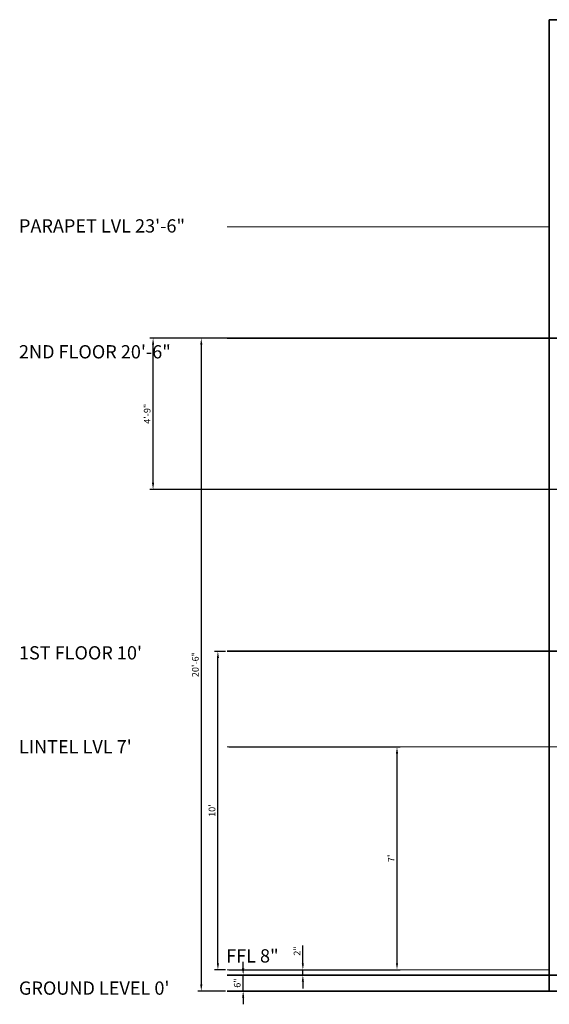
# Model space of a CAD drawing. Units: inches. Extents: x 2443635 to 2446153, y 1826255 to 1827341.
# Tile 12 of 16: x 2444943 to 2445143, y 1826858 to 1827229. Entities that reach past the tile are written whole.
import ezdxf

# ---------------------------------------------------------------- set-up
doc = ezdxf.new("R2010")
doc.units = ezdxf.units.IN
for name, color, linetype, lineweight in [('A-ANNO-LEVL', 4, 'Continuous', 18), ('A-DIMS', 1, 'Continuous', 18), ('A-SECT', 7, 'Continuous', 35)]:
    doc.layers.add(name, color=color, linetype=linetype, lineweight=lineweight)
doc.styles.get("Standard").update_dxf_attribs({"font": 'arial.ttf'})
doc.dimstyles.new('ISO-25', dxfattribs={"dimtxt": 2.5, "dimasz": 2.5, "dimexe": 1.25, "dimexo": 0.625, "dimtad": 1, "dimlunit": 4, "dimtxsty": 'Standard', "dimcen": 2.5, "dimadec": 0, "dimazin": 0, "dimtfac": 1, "dimtmove": 0, "dimatfit": 3, "dimfxl": 1, "dimarcsym": 0})

# ---------------------------------------------------------------- blocks, each defined once
blk = doc.blocks.new('*D31')
at = {"layer": 'A-DIMS', "color": 0, "lineweight": -2, "transparency": 16777216}
for p, q in [((2445027.46, 1826871.2), (2445027.46, 1826873.7)), ((2445022.02, 1826868.7), (2445028.71, 1826868.7)), ((2445027.46, 1826862.7), (2445027.46, 1826868.7)), ((2445022.02, 1826862.7), (2445028.71, 1826862.7)), ((2445027.46, 1826860.2), (2445027.46, 1826857.7))]:
    blk.add_line(p, q, dxfattribs=at)
at = {"layer": 'A-DIMS', "color": 0, "transparency": 16777216}
for points in [[(2445027.04, 1826871.2), (2445027.87, 1826871.2), (2445027.46, 1826868.7)], [(2445027.04, 1826860.2), (2445027.87, 1826860.2), (2445027.46, 1826862.7)]]:
    blk.add_solid(points, dxfattribs=at)
at = {"layer": 'Defpoints', "color": 0, "transparency": 16777216}
for p in [(2445021.4, 1826868.7), (2445027.46, 1826868.7), (2445021.4, 1826862.7)]:
    blk.add_point(p, dxfattribs=at)
at = {"layer": 'A-DIMS', "color": 0, "transparency": 16777216, "insert": (2445025.55, 1826865.7), "char_height": 2.5, "attachment_point": 5, "rotation": 90}
blk.add_mtext('6"', dxfattribs=at)
blk = doc.blocks.new('*D32')
at = {"layer": 'A-DIMS', "color": 0, "lineweight": -2, "transparency": 16777216}
for p, q in [((2445049.96, 1826873.2), (2445049.96, 1826879.87)), ((2445022.02, 1826870.7), (2445051.21, 1826870.7)), ((2445022.02, 1826868.7), (2445051.21, 1826868.7)), ((2445049.96, 1826868.7), (2445049.96, 1826870.7)), ((2445049.96, 1826866.2), (2445049.96, 1826863.7))]:
    blk.add_line(p, q, dxfattribs=at)
at = {"layer": 'A-DIMS', "color": 0, "transparency": 16777216}
for points in [[(2445049.54, 1826873.2), (2445050.37, 1826873.2), (2445049.96, 1826870.7)], [(2445049.54, 1826866.2), (2445050.37, 1826866.2), (2445049.96, 1826868.7)]]:
    blk.add_solid(points, dxfattribs=at)
at = {"layer": 'Defpoints', "color": 0, "transparency": 16777216}
for p in [(2445021.4, 1826870.7), (2445021.4, 1826868.7), (2445049.96, 1826870.7)]:
    blk.add_point(p, dxfattribs=at)
at = {"layer": 'A-DIMS', "color": 0, "transparency": 16777216, "insert": (2445048.08, 1826877.78), "char_height": 2.5, "attachment_point": 5, "rotation": 90}
blk.add_mtext('2"', dxfattribs=at)
blk = doc.blocks.new('*D33')
at = {"layer": 'A-DIMS', "color": 0, "lineweight": -2, "transparency": 16777216}
for p, q in [((2445022.02, 1826954.7), (2445086.7, 1826954.7)), ((2445085.45, 1826873.2), (2445085.45, 1826952.2)), ((2445022.02, 1826870.7), (2445086.7, 1826870.7))]:
    blk.add_line(p, q, dxfattribs=at)
at = {"layer": 'A-DIMS', "color": 0, "transparency": 16777216}
for points in [[(2445085.03, 1826952.2), (2445085.86, 1826952.2), (2445085.45, 1826954.7)], [(2445085.03, 1826873.2), (2445085.86, 1826873.2), (2445085.45, 1826870.7)]]:
    blk.add_solid(points, dxfattribs=at)
at = {"layer": 'Defpoints', "color": 0, "transparency": 16777216}
for p in [(2445021.4, 1826954.7), (2445085.45, 1826954.7), (2445021.4, 1826870.7)]:
    blk.add_point(p, dxfattribs=at)
at = {"layer": 'A-DIMS', "color": 0, "transparency": 16777216, "insert": (2445083.57, 1826912.7), "char_height": 2.5, "attachment_point": 5, "rotation": 90}
blk.add_mtext("7'", dxfattribs=at)
blk = doc.blocks.new('*D34')
at = {"layer": 'A-DIMS', "color": 0, "lineweight": -2, "transparency": 16777216}
for p, q in [((2445020.77, 1826990.7), (2445016.69, 1826990.7)), ((2445017.94, 1826873.2), (2445017.94, 1826988.2)), ((2445020.77, 1826870.7), (2445016.69, 1826870.7))]:
    blk.add_line(p, q, dxfattribs=at)
at = {"layer": 'A-DIMS', "color": 0, "transparency": 16777216}
for points in [[(2445017.53, 1826988.2), (2445018.36, 1826988.2), (2445017.94, 1826990.7)], [(2445017.53, 1826873.2), (2445018.36, 1826873.2), (2445017.94, 1826870.7)]]:
    blk.add_solid(points, dxfattribs=at)
at = {"layer": 'Defpoints', "color": 0, "transparency": 16777216}
for p in [(2445017.94, 1826990.7), (2445021.4, 1826990.7), (2445021.4, 1826870.7)]:
    blk.add_point(p, dxfattribs=at)
at = {"layer": 'A-DIMS', "color": 0, "transparency": 16777216, "insert": (2445016.04, 1826930.7), "char_height": 2.5, "attachment_point": 5, "rotation": 90}
blk.add_mtext("10'", dxfattribs=at)
blk = doc.blocks.new('*D35')
at = {"layer": 'A-DIMS', "color": 0, "lineweight": -2, "transparency": 16777216}
for p, q in [((2445020.77, 1827108.7), (2445010.42, 1827108.7)), ((2445011.67, 1827106.2), (2445011.67, 1826865.2)), ((2445020.77, 1826862.7), (2445010.42, 1826862.7))]:
    blk.add_line(p, q, dxfattribs=at)
at = {"layer": 'A-DIMS', "color": 0, "transparency": 16777216}
for points in [[(2445011.26, 1827106.2), (2445012.09, 1827106.2), (2445011.67, 1827108.7)], [(2445011.26, 1826865.2), (2445012.09, 1826865.2), (2445011.67, 1826862.7)]]:
    blk.add_solid(points, dxfattribs=at)
at = {"layer": 'Defpoints', "color": 0, "transparency": 16777216}
for p in [(2445021.4, 1827108.7), (2445011.67, 1826862.7), (2445021.4, 1826862.7)]:
    blk.add_point(p, dxfattribs=at)
at = {"layer": 'A-DIMS', "color": 0, "transparency": 16777216, "insert": (2445009.77, 1826985.7), "char_height": 2.5, "attachment_point": 5, "rotation": 90}
blk.add_mtext('20\'-6"', dxfattribs=at)
blk = doc.blocks.new('*D104')
at = {"layer": 'A-DIMS', "color": 0, "lineweight": -2, "transparency": 16777216}
for p, q in [((2445256.24, 1827108.7), (2444992.25, 1827108.7)), ((2444993.5, 1827054.2), (2444993.5, 1827106.2)), ((2445193.24, 1827051.7), (2444992.25, 1827051.7))]:
    blk.add_line(p, q, dxfattribs=at)
at = {"layer": 'A-DIMS', "color": 0, "transparency": 16777216}
for points in [[(2444993.08, 1827106.2), (2444993.91, 1827106.2), (2444993.5, 1827108.7)], [(2444993.08, 1827054.2), (2444993.91, 1827054.2), (2444993.5, 1827051.7)]]:
    blk.add_solid(points, dxfattribs=at)
at = {"layer": 'Defpoints', "color": 0, "transparency": 16777216}
for p in [(2444993.5, 1827108.7), (2445256.86, 1827108.7), (2445193.86, 1827051.7)]:
    blk.add_point(p, dxfattribs=at)
at = {"layer": 'A-DIMS', "color": 0, "transparency": 16777216, "insert": (2444991.6, 1827080.2), "char_height": 2.5, "attachment_point": 5, "rotation": 90}
blk.add_mtext('4\'-9"', dxfattribs=at)

msp = doc.modelspace()

# ---------------------------------------------------------------- linework, layer by layer
at = {"layer": 'A-ANNO-LEVL'}
for p, q in [((2445142.864, 1827150.701), (2445021.398, 1827150.701)), ((2445220.864, 1826954.701), (2445021.398, 1826954.701)), ((2445142.864, 1826870.701), (2445021.398, 1826870.701))]:
    msp.add_line(p, q, dxfattribs=at)
at = {"layer": 'A-SECT'}
for p, q in [((2445142.864, 1827228.701), (2445142.864, 1826862.701)), ((2445285.491, 1827228.701), (2445142.864, 1827228.701)), ((2445478.864, 1827108.701), (2445021.398, 1827108.701)), ((2445457.864, 1826990.701), (2445021.398, 1826990.701)), ((2445490.864, 1826868.701), (2445021.398, 1826868.701)), ((2445478.864, 1826862.701), (2445021.398, 1826862.701))]:
    msp.add_line(p, q, dxfattribs=at)

# ---------------------------------------------------------------- texts
at = {"layer": 'A-ANNO-LEVL', "char_height": 5, "attachment_point": 1}
for s, insert in [('PARAPET LVL 23\'-6"', (2444942.948, 1827153.499)), ('2ND FLOOR 20\'-6"', (2444942.948, 1827106.065)), ("1ST FLOOR 10'", (2444942.948, 1826992.634)), ("LINTEL LVL 7'", (2444942.948, 1826957.23)), ('FFL 8"', (2445021.047, 1826878.443)), ("GROUND LEVEL 0'", (2444942.948, 1826866.309))]:
    msp.add_mtext_dynamic_manual_height_columns(s, width=91.16265, gutter_width=12.5, heights=[0], dxfattribs=dict(at, insert=insert))

# ---------------------------------------------------------------- dimensions: what is measured, and where the dimension line sits
at = {"layer": 'A-DIMS', "transparency": 33554687}
dim = msp.add_linear_dim(base=(2444993.498, 1827108.701), p1=(2445193.864, 1827051.701), p2=(2445256.864, 1827108.701), angle=90, dimstyle='ISO-25', override={"dimdec": 1, "dimlfac": 1, "dimrnd": 0, "dimzin": 1, "dimdsep": 46, "dimlunit": 4, "dimfrac": 2}, dxfattribs=at)
dim.commit()
dim.dimension.update_dxf_attribs({"geometry": '*D104', "text_midpoint": (2444991.596, 1827080.201)})
at = {"layer": 'A-DIMS'}
for base, p1, p2, picture, middle in [((2445011.672, 1826862.701), (2445021.398, 1827108.701), (2445021.398, 1826862.701), '*D35', (2445009.771, 1826985.701)), ((2445049.955, 1826870.701), (2445021.398, 1826868.701), (2445021.398, 1826870.701), '*D32', (2445048.075, 1826877.784))]:
    dim = msp.add_linear_dim(base=base, p1=p1, p2=p2, angle=90, dimstyle='ISO-25', override={"dimclrd": 0, "dimclre": 0, "dimclrt": 0}, dxfattribs=at)
    dim.commit()
    dim.dimension.update_dxf_attribs({"geometry": picture, "text_midpoint": middle})
for base, p1, p2, picture, middle in [((2445017.944, 1826990.701), (2445021.398, 1826870.701), (2445021.398, 1826990.701), '*D34', (2445017.944, 1826930.701)), ((2445085.447, 1826954.701), (2445021.398, 1826870.701), (2445021.398, 1826954.701), '*D33', (2445085.447, 1826912.701)), ((2445027.456, 1826868.701), (2445021.398, 1826862.701), (2445021.398, 1826868.701), '*D31', (2445027.456, 1826865.701))]:
    dim = msp.add_linear_dim(base=base, p1=p1, p2=p2, angle=90, dimstyle='ISO-25', override={"dimclrd": 0, "dimclre": 0, "dimclrt": 0}, dxfattribs=at)
    dim.commit()
    dim.dimension.update_dxf_attribs({"geometry": picture, "text_midpoint": middle, "dimtype": 160})

doc.saveas('drawing.dxf')
